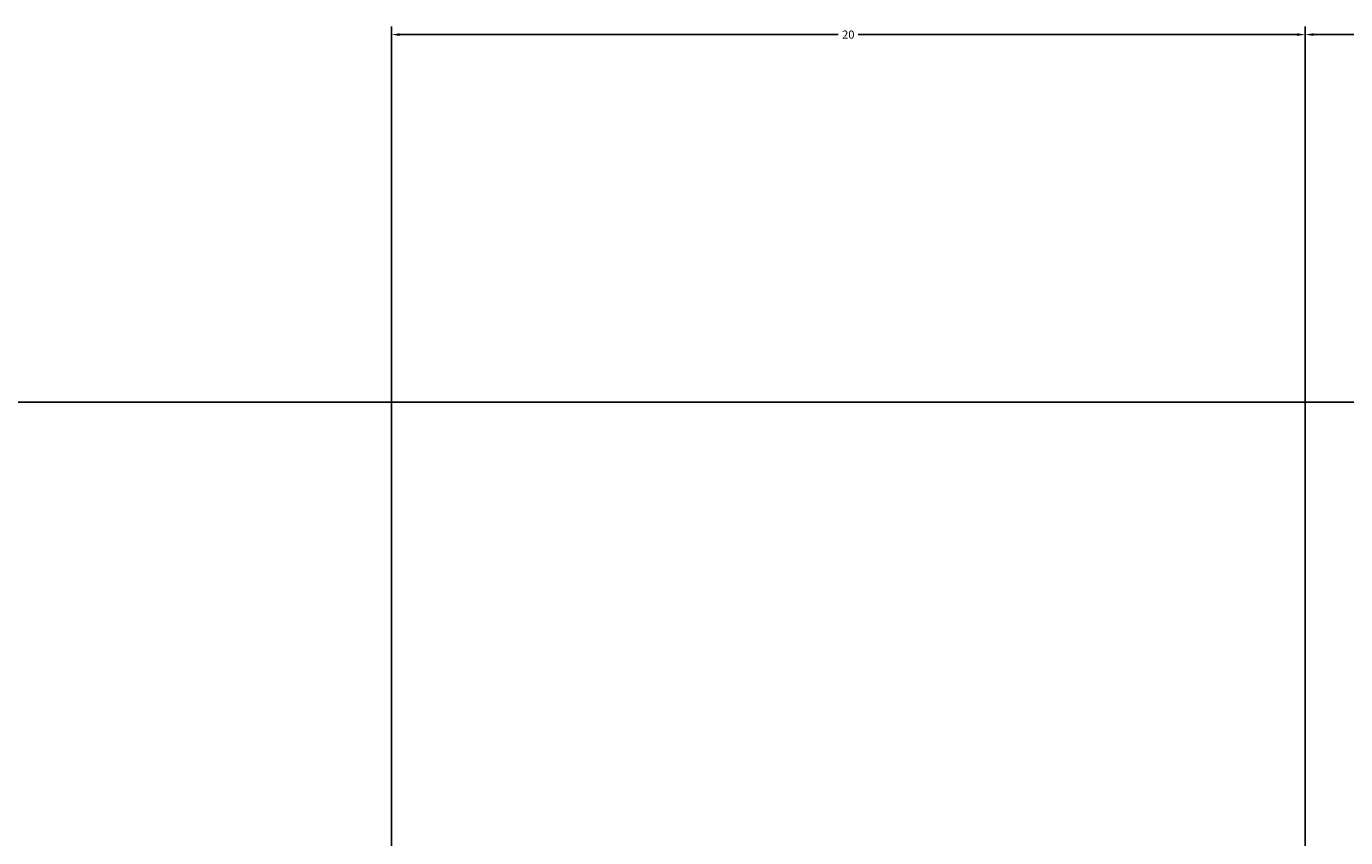
# Model space of a CAD drawing. Units: millimetres. Extents: x -48 to 129, y -118 to -41.
# Tile 4 of 6: x -28 to 1, y -59 to -41. Entities that reach past the tile are written whole.
import ezdxf

# ---------------------------------------------------------------- set-up
doc = ezdxf.new("R2010")
doc.units = ezdxf.units.MM
doc.layers.add('M-DIMS', color=2, linetype='Continuous', lineweight=18)
doc.styles.get("Standard").update_dxf_attribs({"font": 'arial.ttf'})
doc.dimstyles.get("Standard").update_dxf_attribs({"dimtxt": 0.18, "dimasz": 0.18, "dimexe": 0.18, "dimexo": 0.0625, "dimgap": 0.09, "dimtad": 0, "dimtih": 1, "dimtoh": 1, "dimdec": 4, "dimzin": 0, "dimdsep": 46, "dimtxsty": 'Standard', "dimcen": 0.09, "dimadec": 0, "dimazin": 0, "dimtfac": 1, "dimtdec": 4, "dimtofl": 0, "dimtmove": 0, "dimatfit": 3, "dimfxl": 1, "dimtolj": 1, "dimtzin": 0, "dimarcsym": 0})

# ---------------------------------------------------------------- blocks, each defined once
blk = doc.blocks.new('*D2')
at = {"layer": 'Defpoints', "color": 0, "transparency": 16777216}
for p in [(0, -41.392), (0, -59.442), (-20, -79.442)]:
    blk.add_point(p, dxfattribs=at)
at = {"layer": 'M-DIMS', "color": 0, "lineweight": -2, "transparency": 16777216}
for p, q in [((-20, -79.38), (-20, -41.212)), ((0, -59.38), (0, -41.212)), ((-19.82, -41.392), (-10.22, -41.392)), ((-0.18, -41.392), (-9.78, -41.392))]:
    blk.add_line(p, q, dxfattribs=at)
at = {"layer": 'M-DIMS', "color": 0, "transparency": 16777216}
for points in [[(-19.82, -41.362), (-19.82, -41.422), (-20, -41.392)], [(-0.18, -41.362), (-0.18, -41.422), (0, -41.392)]]:
    blk.add_solid(points, dxfattribs=at)
at = {"layer": 'M-DIMS', "color": 0, "transparency": 16777216, "insert": (-10, -41.392), "char_height": 0.18, "attachment_point": 5}
blk.add_mtext('\\A1;20', dxfattribs=at)
blk = doc.blocks.new('*D3')
at = {"layer": 'Defpoints', "color": 0, "transparency": 16777216}
for p in [(90, -41.392), (0, -59.442), (90, -79.442)]:
    blk.add_point(p, dxfattribs=at)
at = {"layer": 'M-DIMS', "color": 0, "lineweight": -2, "transparency": 16777216}
for p, q in [((0, -59.38), (0, -41.212)), ((90, -79.38), (90, -41.212)), ((0.18, -41.392), (44.781, -41.392)), ((89.82, -41.392), (45.219, -41.392))]:
    blk.add_line(p, q, dxfattribs=at)
at = {"layer": 'M-DIMS', "color": 0, "transparency": 16777216}
for points in [[(0.18, -41.362), (0.18, -41.422), (0, -41.392)], [(89.82, -41.362), (89.82, -41.422), (90, -41.392)]]:
    blk.add_solid(points, dxfattribs=at)
at = {"layer": 'M-DIMS', "color": 0, "transparency": 16777216, "insert": (45, -41.392), "char_height": 0.18, "attachment_point": 5}
blk.add_mtext('\\A1;90', dxfattribs=at)
blk = doc.blocks.new('*D8')
at = {"layer": 'Defpoints', "color": 0, "transparency": 16777216}
for p in [(-48.05, -49.442), (90, -49.442), (0, -59.442)]:
    blk.add_point(p, dxfattribs=at)
at = {"layer": 'M-DIMS', "color": 0, "lineweight": -2, "transparency": 16777216}
for p, q in [((89.938, -49.442), (-48.23, -49.442)), ((-48.05, -49.622), (-48.05, -54.26)), ((-48.05, -59.262), (-48.05, -54.624)), ((-0.062, -59.442), (-48.23, -59.442))]:
    blk.add_line(p, q, dxfattribs=at)
at = {"layer": 'M-DIMS', "color": 0, "transparency": 16777216}
for points in [[(-48.08, -49.622), (-48.02, -49.622), (-48.05, -49.442)], [(-48.08, -59.262), (-48.02, -59.262), (-48.05, -59.442)]]:
    blk.add_solid(points, dxfattribs=at)
at = {"layer": 'M-DIMS', "color": 0, "transparency": 16777216, "insert": (-48.05, -54.442), "char_height": 0.18, "attachment_point": 5}
blk.add_mtext('\\A1;10', dxfattribs=at)

msp = doc.modelspace()

# ---------------------------------------------------------------- dimensions: what is measured, and where the dimension line sits
at = {"layer": 'M-DIMS'}
for base, p1, p2, picture, middle in [((0, -41.392), (-20, -79.442), (0, -59.442), '*D2', (-10, -41.392)), ((90, -41.392), (0, -59.442), (90, -79.442), '*D3', (45, -41.392))]:
    dim = msp.add_linear_dim(base=base, p1=p1, p2=p2, dimstyle='Standard', override={"dimdec": 0, "dimlfac": 1, "dimrnd": 0, "dimzin": 0, "dimdsep": 46, "dimlunit": 2}, dxfattribs=at)
    dim.commit()
    dim.dimension.update_dxf_attribs({"geometry": picture, "text_midpoint": middle})
dim = msp.add_linear_dim(base=(-48.05, -49.442), p1=(0, -59.442), p2=(90, -49.442), angle=90, dimstyle='Standard', override={"dimdec": 0, "dimlfac": 1, "dimrnd": 0, "dimzin": 0, "dimdsep": 46, "dimlunit": 2}, dxfattribs=at)
dim.commit()
dim.dimension.update_dxf_attribs({"geometry": '*D8', "text_midpoint": (-48.05, -54.442)})

doc.saveas('drawing.dxf')
